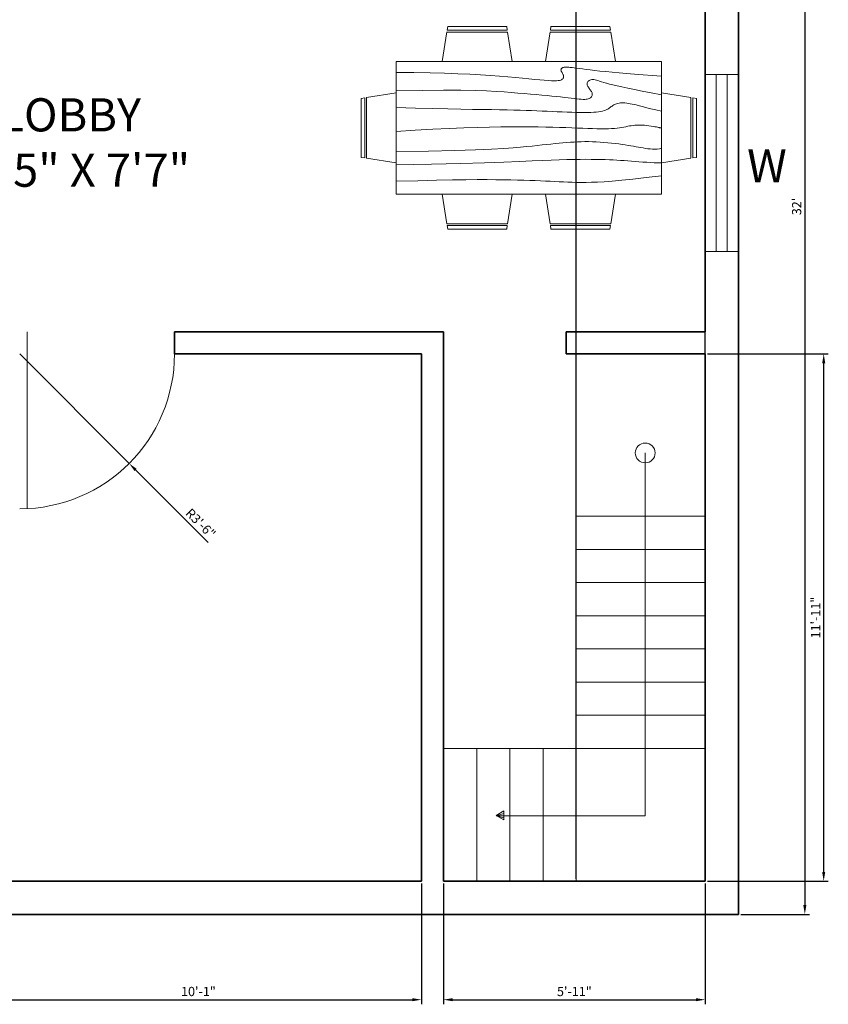
# Model space of a CAD drawing. Units: inches. Extents: x 1642 to 5612, y 1595 to 4064.
# Tile 5 of 6: x 2539 to 2759, y 1712 to 1979. Entities that reach past the tile are written whole.
import ezdxf

# ---------------------------------------------------------------- set-up
doc = ezdxf.new("R2010")
doc.units = ezdxf.units.IN
for name, color, linetype, lineweight in [('A-ANNO-DIMS', 2, 'Continuous', 18), ('A-ANNO-SYMB', 2, 'Continuous', 13), ('A-ANNO-TEXT', 7, 'Continuous', 18), ('A-AREA-IDEN', 7, 'Continuous', 25), ('A-DOOR', 3, 'Continuous', 18), ('A-FLOR-STRS', 7, 'Continuous', 18), ('A-FURN', 8, 'Continuous', 13), ('A-GLAZ', 4, 'Continuous', 18), ('A-WALL', 7, 'Continuous', 35)]:
    doc.layers.add(name, color=color, linetype=linetype, lineweight=lineweight)
doc.styles.get("Standard").update_dxf_attribs({"font": 'arial.ttf'})
doc.dimstyles.new('ISO-25', dxfattribs={"dimtxt": 2.5, "dimasz": 2.5, "dimexe": 1.25, "dimexo": 0.625, "dimtad": 1, "dimdec": 0, "dimlunit": 3, "dimtxsty": 'Standard', "dimcen": 2.5, "dimadec": 0, "dimazin": 0, "dimtfac": 1, "dimtdec": 0, "dimtmove": 0, "dimatfit": 3, "dimfxl": 1, "dimarcsym": 0})

# ---------------------------------------------------------------- blocks, each defined once
blk = doc.blocks.new('Dining Set - 36 x 72 in.')
for p, q in [((-22, 27.5), (-22.1562, 26.50042)), ((-22, 27.5), (-6, 27.5)), ((-5.8437, 26.49966), (-6, 27.5)), ((6, 27.5), (5.8438, 26.50042)), ((6, 27.5), (22, 27.5)), ((22.1563, 26.49966), (22, 27.5)), ((-22.2343, 26.00059), (-23.4847, 17.99762)), ((-22.2304, 26), (-5.7608, 26)), ((-5.8416, 26.5), (-22.1534, 26.5)), ((-4.5152, 17.99762), (-5.7655, 25.99926)), ((5.7657, 26.00059), (4.5153, 17.99762)), ((5.7696, 26), (22.2392, 26)), ((22.1584, 26.5), (5.8466, 26.5)), ((23.4848, 17.99762), (22.2345, 25.99926)), ((36, 18), (-36, 18)), ((-36, 18), (-36, -18)), ((36, -18), (36, 18)), ((-45.5, 8), (-44.5004, 8.15617)), ((-44.5, -8.15843), (-44.5, 8.15338)), ((-44.0006, 8.23428), (-35.9976, 9.48474)), ((-44, 8.23041), (-44, -8.23915)), ((44.0006, 8.23428), (35.9976, 9.48474)), ((44, 8.23041), (44, -8.23915)), ((44.5, -8.15843), (44.5, 8.15338)), ((45.5, 8), (44.5005, 8.15617)), ((-45.5, 8), (-45.5, -8)), ((45.5, 8), (45.5, -8)), ((-44.4997, -8.15631), (-45.5, -8)), ((44.4997, -8.15631), (45.5, -8)), ((-35.9976, -9.48476), (-43.9993, -8.2345)), ((35.9976, -9.48476), (43.9993, -8.2345)), ((-36, -18), (36, -18)), ((-22.2343, -26.0006), (-23.4847, -17.99762)), ((-4.5152, -17.99762), (-5.7655, -25.99928)), ((5.7657, -26.0006), (4.5153, -17.99762)), ((23.4848, -17.99762), (22.2345, -25.99928)), ((-22.2304, -26), (-5.7608, -26)), ((-22, -27.5), (-22.1562, -26.50044)), ((-5.8416, -26.5), (-22.1534, -26.5)), ((-5.8437, -26.49967), (-6, -27.5)), ((5.7696, -26), (22.2392, -26)), ((6, -27.5), (5.8438, -26.50044)), ((22.1584, -26.5), (5.8466, -26.5)), ((22.1563, -26.49967), (22, -27.5)), ((-22, -27.5), (-6, -27.5)), ((6, -27.5), (22, -27.5))]:
    blk.add_line(p, q)
for points in [[(-36, 15), (-31.1772, 14.97754), (-26.8079, 14.91406), (-22.8538, 14.81543), (-19.276, 14.6875), (-16.0362, 14.53613), (-13.0957, 14.36718), (-10.4159, 14.18652), (-7.9583, 14), (-5.6904, 13.81315), (-3.6035, 13.63021), (-1.6954, 13.45508), (0.0365, 13.29166), (1.5945, 13.14388), (2.9811, 13.01562), (4.1988, 12.9108), (5.25, 12.83333), (6.1393, 12.78613), (6.8802, 12.76823), (7.4883, 12.77767), (7.9792, 12.8125), (8.3685, 12.87077), (8.6719, 12.95052), (8.9049, 13.0498), (9.0833, 13.16666), (9.2205, 13.29899), (9.3216, 13.44401), (9.3895, 13.59879), (9.4271, 13.76041), (9.4373, 13.92594), (9.4232, 14.09245), (9.3875, 14.257), (9.3333, 14.41666), (9.2638, 14.56917), (9.1836, 14.71484), (9.0975, 14.85465), (9.0104, 14.98958), (8.9272, 15.1206), (8.8529, 15.2487), (8.7922, 15.37483), (8.75, 15.5), (8.7305, 15.62467), (8.7344, 15.74739), (8.7617, 15.86621), (8.8125, 15.97916), (8.8867, 16.08431), (8.9844, 16.17968), (9.1055, 16.26334), (9.25, 16.33333), (9.4189, 16.38802), (9.6172, 16.42708), (9.8506, 16.45052), (10.125, 16.45833), (10.4463, 16.45052), (10.8203, 16.42708), (11.2529, 16.38802), (11.75, 16.33333), (12.3184, 16.26318), (12.9694, 16.17838), (13.7151, 16.07991), (14.5677, 15.96875), (15.5395, 15.84586), (16.6426, 15.71224), (17.8893, 15.56884), (19.2917, 15.41666), (20.859, 15.25667), (22.5879, 15.08984), (24.4721, 14.91715), (26.5052, 14.73958), (28.6809, 14.5581), (30.9929, 14.3737), (33.4347, 14.18733), (36, 14)], [(-36, 10), (-28.9766, 10.14274), (-23.1725, 10.20442), (-18.4241, 10.19775), (-14.5677, 10.13541), (-11.4399, 10.03011), (-8.877, 9.89453), (-6.7154, 9.74137), (-4.7917, 9.58333), (-2.9698, 9.43082), (-1.2246, 9.28515), (0.4415, 9.14534), (2.026, 9.01041), (3.5266, 8.87939), (4.9408, 8.7513), (6.266, 8.62516), (7.5, 8.5), (8.6411, 8.37549), (9.6914, 8.2539), (10.6538, 8.13818), (11.5312, 8.03125), (12.3267, 7.93603), (13.043, 7.85547), (13.6831, 7.79248), (14.25, 7.75), (14.7471, 7.7303), (15.1797, 7.73307), (15.5537, 7.75732), (15.875, 7.80208), (16.1494, 7.86637), (16.3828, 7.94922), (16.5811, 8.04964), (16.75, 8.16666), (16.8944, 8.29915), (17.0143, 8.44531), (17.1089, 8.60319), (17.1771, 8.77083), (17.218, 8.94629), (17.2305, 9.1276), (17.2137, 9.31282), (17.1667, 9.5), (17.0895, 9.6875), (16.987, 9.875), (16.8649, 10.0625), (16.7292, 10.25), (16.5856, 10.4375), (16.4401, 10.625), (16.2985, 10.8125), (16.1667, 11), (16.05, 11.18733), (15.9518, 11.3737), (15.8752, 11.5581), (15.8229, 11.73958), (15.798, 11.91715), (15.8034, 12.08984), (15.842, 12.25667), (15.9167, 12.41666), (16.0295, 12.56836), (16.1784, 12.70833), (16.3605, 12.83268), (16.5729, 12.9375), (16.8127, 13.01888), (17.0768, 13.07291), (17.3625, 13.0957), (17.6667, 13.08333), (17.9894, 13.03312), (18.3418, 12.94726), (18.7382, 12.82918), (19.1927, 12.68229), (19.7195, 12.51001), (20.3327, 12.31575), (21.0465, 12.10294), (21.875, 11.875), (22.8357, 11.63354), (23.959, 11.37304), (25.2786, 11.08618), (26.8282, 10.76562), (28.6414, 10.40405), (30.752, 9.99414), (33.1936, 9.52856), (36, 9)], [(-36, 5.5), (-30.7157, 5.3348), (-26.069, 5.20963), (-21.9946, 5.11767), (-18.4271, 5.05208), (-15.3009, 5.00602), (-12.5508, 4.97265), (-10.1112, 4.94515), (-7.9167, 4.91666), (-5.909, 4.88167), (-4.0586, 4.83984), (-2.3429, 4.79215), (-0.7396, 4.73958), (0.7739, 4.6831), (2.22, 4.6237), (3.6213, 4.56233), (5, 4.5), (6.373, 4.43782), (7.7344, 4.3776), (9.0723, 4.32129), (10.375, 4.27083), (11.6309, 4.22819), (12.8281, 4.19531), (13.9551, 4.17415), (15, 4.16666), (15.954, 4.17448), (16.819, 4.19791), (17.6001, 4.23698), (18.3021, 4.29166), (18.9299, 4.36198), (19.4883, 4.44791), (19.9823, 4.54948), (20.4167, 4.66666), (20.7969, 4.79899), (21.1302, 4.94401), (21.4245, 5.09879), (21.6875, 5.26041), (21.9271, 5.42594), (22.1511, 5.59245), (22.3672, 5.757), (22.5834, 5.91666), (22.8065, 6.06868), (23.0404, 6.21093), (23.2879, 6.34147), (23.5521, 6.45833), (23.8358, 6.55957), (24.142, 6.64323), (24.4735, 6.70735), (24.8334, 6.75), (25.2235, 6.76969), (25.642, 6.76692), (26.0858, 6.74267), (26.5521, 6.69791), (27.0379, 6.63362), (27.5404, 6.55078), (28.0565, 6.45036), (28.5834, 6.33333), (29.1242, 6.19987), (29.7071, 6.04687), (30.3661, 5.87044), (31.1354, 5.66666), (32.0493, 5.43164), (33.142, 5.16146), (34.4475, 4.85221), (36, 4.5)], [(-36, -1), (-30.7915, -0.6591), (-26.0195, -0.38216), (-21.6519, -0.16284), (-17.6563, 0.00521), (-14.0005, 0.12833), (-10.6523, 0.21289), (-7.5796, 0.26522), (-4.75, 0.29166), (-2.134, 0.29793), (0.2878, 0.28711), (2.5317, 0.26163), (4.6146, 0.22396), (6.5529, 0.17651), (8.3633, 0.12174), (10.0623, 0.06209), (11.6667, 0), (13.1899, -0.06201), (14.6341, -0.1211), (15.9982, -0.17432), (17.2813, -0.21875), (18.4823, -0.25147), (19.6003, -0.26953), (20.6343, -0.27002), (21.5834, -0.25), (22.4481, -0.20768), (23.2357, -0.14584), (23.9549, -0.06836), (24.6146, 0.02083), (25.2235, 0.11784), (25.7904, 0.21875), (26.3241, 0.31966), (26.8334, 0.41666), (27.3265, 0.50618), (27.8099, 0.58593), (28.2894, 0.65397), (28.7709, 0.70833), (29.2601, 0.74707), (29.763, 0.76823), (30.2855, 0.76985), (30.8334, 0.75), (31.4088, 0.70784), (31.9994, 0.64713), (32.589, 0.57275), (33.1615, 0.48958), (33.7008, 0.4025), (34.1908, 0.3164), (34.6153, 0.23616), (34.9584, 0.16666), (35.2099, 0.11165), (35.3848, 0.07031), (35.504, 0.04069), (35.5886, 0.02083), (35.6594, 0.00879), (35.7377, 0.0026), (35.8442, 0.00032), (36, 0)], [(-36, -6.5), (-27.1843, -6.31267), (-20.084, -6.1263), (-14.469, -5.9419), (-10.1094, -5.76042), (-6.7752, -5.58285), (-4.2363, -5.41016), (-2.2629, -5.24333), (-0.625, -5.08334), (0.8708, -4.93099), (2.2715, -4.78646), (3.5872, -4.64974), (4.8281, -4.52084), (6.0046, -4.39974), (7.127, -4.28646), (8.2053, -4.18099), (9.25, -4.08334), (10.2705, -3.99382), (11.2734, -3.91407), (12.2647, -3.84603), (13.25, -3.79167), (14.2354, -3.75293), (15.2266, -3.73177), (16.2295, -3.73015), (17.25, -3.75), (18.2912, -3.79248), (19.3451, -3.85547), (20.4009, -3.93604), (21.4479, -4.03125), (22.4754, -4.13819), (23.4727, -4.25391), (24.4289, -4.37549), (25.3334, -4.5), (26.1785, -4.62492), (26.9694, -4.74935), (27.7145, -4.87281), (28.4219, -4.99479), (29.1, -5.11483), (29.7572, -5.23242), (30.4016, -5.34709), (31.0417, -5.45834), (31.6837, -5.56437), (32.3262, -5.65821), (32.9658, -5.73153), (33.599, -5.77604), (34.2224, -5.78345), (34.8327, -5.74545), (35.4264, -5.65373), (36, -5.5)], [(-36, -10), (-26.4022, -9.81299), (-18.4675, -9.62891), (-11.9839, -9.45069), (-6.7396, -9.28125), (-2.5226, -9.12354), (0.8789, -8.98047), (3.6769, -8.85498), (6.0833, -8.75), (8.2767, -8.66765), (10.3021, -8.60677), (12.1712, -8.56543), (13.8958, -8.54167), (15.4876, -8.53353), (16.9583, -8.53907), (18.3197, -8.55632), (19.5834, -8.58334), (20.7616, -8.61841), (21.8685, -8.66081), (22.9188, -8.71004), (23.9271, -8.76563), (24.9081, -8.82707), (25.8763, -8.89388), (26.8465, -8.96558), (27.8334, -9.04167), (28.8474, -9.12118), (29.8828, -9.20117), (30.93, -9.27824), (31.9792, -9.34896), (33.0205, -9.40991), (34.0443, -9.45768), (35.0407, -9.48885), (36, -9.5)], [(-36, -14.5), (-30.0881, -14.33513), (-25.0332, -14.21224), (-20.7312, -14.12647), (-17.0781, -14.07292), (-13.97, -14.04671), (-11.3027, -14.04297), (-8.9724, -14.05681), (-6.875, -14.08334), (-4.9224, -14.11833), (-3.0905, -14.16016), (-1.3709, -14.20785), (0.2448, -14.26042), (1.7647, -14.3169), (3.1973, -14.3763), (4.5507, -14.43767), (5.8333, -14.5), (7.0554, -14.5621), (8.235, -14.62175), (9.3922, -14.67652), (10.5469, -14.72396), (11.7192, -14.76164), (12.929, -14.78711), (14.1965, -14.79794), (15.5417, -14.79167), (16.9933, -14.76424), (18.6152, -14.70508), (20.4804, -14.60197), (22.6615, -14.44271), (25.2312, -14.21509), (28.2624, -13.9069), (31.8277, -13.50594), (36, -13)]]:
    blk.add_lwpolyline(points)
blk = doc.blocks.new('*D15')
at = {"layer": 'A-ANNO-DIMS', "color": 0, "lineweight": -2, "transparency": 16777216}
for p, q in [((2734.9, 2120.64), (2753.55, 2120.64)), ((2752.3, 2118.14), (2752.3, 1739.14)), ((2734.9, 1736.64), (2753.55, 1736.64))]:
    blk.add_line(p, q, dxfattribs=at)
at = {"layer": 'A-ANNO-DIMS', "color": 0, "transparency": 16777216}
for points in [[(2751.88, 2118.14), (2752.72, 2118.14), (2752.3, 2120.64)], [(2751.88, 1739.14), (2752.72, 1739.14), (2752.3, 1736.64)]]:
    blk.add_solid(points, dxfattribs=at)
at = {"layer": 'Defpoints', "color": 0, "transparency": 16777216}
for p in [(2734.27, 2120.64), (2734.27, 1736.64), (2752.3, 1736.64)]:
    blk.add_point(p, dxfattribs=at)
at = {"layer": 'A-ANNO-DIMS', "color": 0, "transparency": 16777216, "insert": (2750.4, 1928.64), "char_height": 2.5, "attachment_point": 5, "rotation": 90}
blk.add_mtext("32'", dxfattribs=at)
blk = doc.blocks.new('WIN-48x9')
for p, q in [((0, 48), (0, 0)), ((9, 48), (0, 48)), ((3, 48), (3, 0)), ((6, 0), (6, 48)), ((9, 0), (9, 48)), ((0, 0), (9, 0))]:
    blk.add_line(p, q)
blk = doc.blocks.new('*D56')
at = {"layer": 'A-ANNO-DIMS', "color": 0, "lineweight": -2, "transparency": 16777216}
for p, q in [((2527.27, 1745.01), (2527.27, 1712.24)), ((2648.27, 1745.01), (2648.27, 1712.24)), ((2529.77, 1713.49), (2645.77, 1713.49))]:
    blk.add_line(p, q, dxfattribs=at)
at = {"layer": 'A-ANNO-DIMS', "color": 0, "transparency": 16777216}
for points in [[(2529.77, 1713.9), (2529.77, 1713.07), (2527.27, 1713.49)], [(2645.77, 1713.9), (2645.77, 1713.07), (2648.27, 1713.49)]]:
    blk.add_solid(points, dxfattribs=at)
at = {"layer": 'Defpoints', "color": 0, "transparency": 16777216}
for p in [(2527.27, 1745.64), (2648.27, 1745.64), (2648.27, 1713.49)]:
    blk.add_point(p, dxfattribs=at)
at = {"layer": 'A-ANNO-DIMS', "color": 0, "transparency": 16777216, "insert": (2587.77, 1715.39), "char_height": 2.5, "attachment_point": 5}
blk.add_mtext('10\'-1"', dxfattribs=at)
blk = doc.blocks.new('*D57')
at = {"layer": 'A-ANNO-DIMS', "color": 0, "lineweight": -2, "transparency": 16777216}
for p, q in [((2654.27, 1745.01), (2654.27, 1712.24)), ((2725.27, 1745.01), (2725.27, 1712.24)), ((2656.77, 1713.49), (2722.77, 1713.49))]:
    blk.add_line(p, q, dxfattribs=at)
at = {"layer": 'A-ANNO-DIMS', "color": 0, "transparency": 16777216}
for points in [[(2656.77, 1713.9), (2656.77, 1713.07), (2654.27, 1713.49)], [(2722.77, 1713.9), (2722.77, 1713.07), (2725.27, 1713.49)]]:
    blk.add_solid(points, dxfattribs=at)
at = {"layer": 'Defpoints', "color": 0, "transparency": 16777216}
for p in [(2654.27, 1745.64), (2725.27, 1745.64), (2725.27, 1713.49)]:
    blk.add_point(p, dxfattribs=at)
at = {"layer": 'A-ANNO-DIMS', "color": 0, "transparency": 16777216, "insert": (2689.77, 1715.39), "char_height": 2.5, "attachment_point": 5}
blk.add_mtext('5\'-11"', dxfattribs=at)
blk = doc.blocks.new('*D59')
at = {"layer": 'A-ANNO-DIMS', "color": 0, "lineweight": -2, "transparency": 16777216}
for p, q in [((2725.9, 1888.64), (2758.67, 1888.64)), ((2757.42, 1748.14), (2757.42, 1886.14)), ((2725.9, 1745.64), (2758.67, 1745.64))]:
    blk.add_line(p, q, dxfattribs=at)
at = {"layer": 'A-ANNO-DIMS', "color": 0, "transparency": 16777216}
for points in [[(2757.01, 1886.14), (2757.84, 1886.14), (2757.42, 1888.64)], [(2757.01, 1748.14), (2757.84, 1748.14), (2757.42, 1745.64)]]:
    blk.add_solid(points, dxfattribs=at)
at = {"layer": 'Defpoints', "color": 0, "transparency": 16777216}
for p in [(2725.27, 1888.64), (2757.42, 1888.64), (2725.27, 1745.64)]:
    blk.add_point(p, dxfattribs=at)
at = {"layer": 'A-ANNO-DIMS', "color": 0, "transparency": 16777216, "insert": (2755.54, 1817.14), "char_height": 2.5, "attachment_point": 5, "rotation": 90}
blk.add_mtext('11\'-11"', dxfattribs=at)
blk = doc.blocks.new('*D65')
at = {"layer": 'A-ANNO-DIMS', "color": 0, "lineweight": -2, "transparency": 16777216}
for p, q in [((2690.27, 1746.26), (2690.27, 2145.04)), ((2725.27, 1746.26), (2725.27, 2145.04)), ((2692.77, 2143.79), (2722.77, 2143.79))]:
    blk.add_line(p, q, dxfattribs=at)
at = {"layer": 'A-ANNO-DIMS', "color": 0, "transparency": 16777216}
for points in [[(2692.77, 2144.2), (2692.77, 2143.37), (2690.27, 2143.79)], [(2722.77, 2144.2), (2722.77, 2143.37), (2725.27, 2143.79)]]:
    blk.add_solid(points, dxfattribs=at)
at = {"layer": 'Defpoints', "color": 0, "transparency": 16777216}
for p in [(2725.27, 2143.79), (2690.27, 1745.64), (2725.27, 1745.64)]:
    blk.add_point(p, dxfattribs=at)
at = {"layer": 'A-ANNO-DIMS', "color": 0, "transparency": 16777216, "insert": (2707.77, 2145.67), "char_height": 2.5, "attachment_point": 5}
blk.add_mtext('2\'-11"', dxfattribs=at)
blk = doc.blocks.new('*D67')
at = {"layer": 'A-ANNO-DIMS', "color": 0, "lineweight": -2, "transparency": 16777216}
for p, q in [((2539.27, 1888.64), (2568.97, 1858.94)), ((2590.43, 1837.48), (2570.74, 1857.17))]:
    blk.add_line(p, q, dxfattribs=at)
at = {"layer": 'A-ANNO-DIMS', "color": 0, "transparency": 16777216}
blk.add_solid([(2571.03, 1857.46), (2570.44, 1856.88), (2568.97, 1858.94)], dxfattribs=at)
at = {"layer": 'Defpoints', "color": 0, "transparency": 16777216}
for p in [(2539.27, 1888.64), (2568.97, 1858.94)]:
    blk.add_point(p, dxfattribs=at)
at = {"layer": 'A-ANNO-DIMS', "color": 0, "transparency": 16777216, "insert": (2588.14, 1842.46), "char_height": 2.5, "attachment_point": 5, "rotation": 315.0002}
blk.add_mtext('R3\'-6"', dxfattribs=at)

msp = doc.modelspace()

# ---------------------------------------------------------------- linework, layer by layer
at = {"layer": 'A-ANNO-SYMB'}
for p, q in [((2708.99, 1861.79), (2708.99, 1763.39)), ((2668.51, 1763.42), (2670.64, 1764.68)), ((2670.64, 1762.29), (2668.51, 1763.42)), ((2668.57, 1763.39), (2670.64, 1764.03)), ((2670.64, 1763.39), (2668.57, 1763.39)), ((2670.64, 1762.83), (2668.57, 1763.39)), ((2670.64, 1763.39), (2670.64, 1764.68)), ((2670.64, 1764.68), (2670.64, 1762.29)), ((2670.64, 1764.68), (2670.64, 1763.39)), ((2670.64, 1764.03), (2670.64, 1762.83)), ((2708.99, 1763.39), (2670.64, 1763.39))]:
    msp.add_line(p, q, dxfattribs=at)
msp.add_circle((2708.99, 1861.79), 2.69, dxfattribs=at)
at = {"layer": 'A-DOOR'}
for q in [(2541.27, 1894.64), (2541.27, 1846.64)]:
    msp.add_line((2541.27, 1888.64), q, dxfattribs=at)
msp.add_arc((2539.27, 1888.64), 42, 270, 360, dxfattribs=at)
at = {"layer": 'A-FLOR-STRS'}
for p, q in [((2690.27, 1888.64), (2690.27, 1745.64)), ((2690.27, 1844.64), (2725.27, 1844.64)), ((2690.27, 1835.64), (2725.27, 1835.64)), ((2690.27, 1826.64), (2725.27, 1826.64)), ((2690.27, 1817.64), (2725.27, 1817.64)), ((2690.27, 1808.64), (2725.27, 1808.64)), ((2690.27, 1799.64), (2725.27, 1799.64)), ((2690.27, 1790.64), (2725.27, 1790.64)), ((2654.27, 1781.64), (2725.27, 1781.64)), ((2663.27, 1781.64), (2663.27, 1745.64)), ((2672.27, 1781.64), (2672.27, 1745.64)), ((2681.27, 1781.64), (2681.27, 1745.64))]:
    msp.add_line(p, q, dxfattribs=at)
at = {"layer": 'A-WALL'}
for p, q in [((2734.27, 1736.64), (2734.27, 2120.64)), ((2725.27, 1894.64), (2725.27, 1985.64)), ((2581.27, 1894.64), (2581.27, 1888.64)), ((2654.27, 1894.64), (2581.27, 1894.64)), ((2654.27, 1888.64), (2654.27, 1894.64)), ((2725.27, 1894.64), (2687.59, 1894.64)), ((2687.59, 1894.64), (2687.59, 1888.64)), ((2648.27, 1888.64), (2581.27, 1888.64)), ((2648.27, 1888.64), (2648.27, 1745.64)), ((2654.27, 1888.64), (2654.27, 1745.64)), ((2725.27, 1888.64), (2687.59, 1888.64)), ((2725.27, 1745.64), (2725.27, 1888.64)), ((2521.27, 1745.64), (2648.27, 1745.64)), ((2654.27, 1745.64), (2725.27, 1745.64)), ((2362.27, 1736.64), (2734.27, 1736.64))]:
    msp.add_line(p, q, dxfattribs=at)

# ---------------------------------------------------------------- block references
at = {"layer": 'A-FURN'}
msp.add_blockref('Dining Set - 36 x 72 in.', (2677.41, 1949.97), dxfattribs=at)
at = {"layer": 'A-GLAZ'}
msp.add_blockref('WIN-48x9', (2725.27, 1916.47), dxfattribs=at)

# ---------------------------------------------------------------- texts
at = {"layer": 'A-ANNO-TEXT', "insert": (2680.63, 1944.18), "char_height": 9, "attachment_point": 1}
msp.add_mtext_dynamic_manual_height_columns('\\pxqc;W', width=122.7897, gutter_width=12.5, heights=[0], dxfattribs=at)
at = {"layer": 'A-AREA-IDEN', "insert": (2519.81, 1958), "char_height": 9, "attachment_point": 1}
msp.add_mtext_dynamic_manual_height_columns('\\pxqc;LOBBY\\P11\'5" X 7\'7"', width=66.3551, gutter_width=12.5, heights=[0], dxfattribs=at)

# ---------------------------------------------------------------- dimensions: what is measured, and where the dimension line sits
at = {"layer": 'A-ANNO-DIMS'}
for base, p1, p2, picture, middle in [((2725.27, 2143.79), (2690.27, 1745.64), (2725.27, 1745.64), '*D65', (2707.77, 2145.67)), ((2648.27, 1713.49), (2527.27, 1745.64), (2648.27, 1745.64), '*D56', (2587.77, 1715.39)), ((2725.27, 1713.49), (2654.27, 1745.64), (2725.27, 1745.64), '*D57', (2689.77, 1715.39))]:
    dim = msp.add_linear_dim(base=base, p1=p1, p2=p2, dimstyle='ISO-25', override={"dimdec": 1, "dimlfac": 1, "dimrnd": 0, "dimzin": 1, "dimdsep": 46, "dimlunit": 4, "dimfrac": 2}, dxfattribs=at)
    dim.commit()
    dim.dimension.update_dxf_attribs({"geometry": picture, "text_midpoint": middle})
for base, p1, p2, override, picture, middle in [((2752.3, 1736.64), (2734.27, 2120.64), (2734.27, 1736.64), {"dimclrd": 0, "dimclre": 0, "dimclrt": 0}, '*D15', (2750.4, 1928.64)), ((2757.42, 1888.64), (2725.27, 1745.64), (2725.27, 1888.64), {"dimdec": 1, "dimlfac": 1, "dimrnd": 0, "dimzin": 1, "dimdsep": 46, "dimlunit": 4, "dimfrac": 2}, '*D59', (2755.54, 1817.14))]:
    dim = msp.add_linear_dim(base=base, p1=p1, p2=p2, angle=90, dimstyle='ISO-25', override=override, dxfattribs=at)
    dim.commit()
    dim.dimension.update_dxf_attribs({"geometry": picture, "text_midpoint": middle})
dim = msp.add_radius_dim(center=(2539.27, 1888.64), mpoint=(2568.97, 1858.94), dimstyle='ISO-25', override={"dimdec": 1, "dimlfac": 1, "dimrnd": 0, "dimzin": 1, "dimdsep": 46, "dimlunit": 4, "dimfrac": 2}, dxfattribs=at)
dim.commit()
dim.dimension.update_dxf_attribs({"geometry": '*D67', "text_midpoint": (2586.79, 1841.12), "dimtype": 164})

doc.saveas('drawing.dxf')
